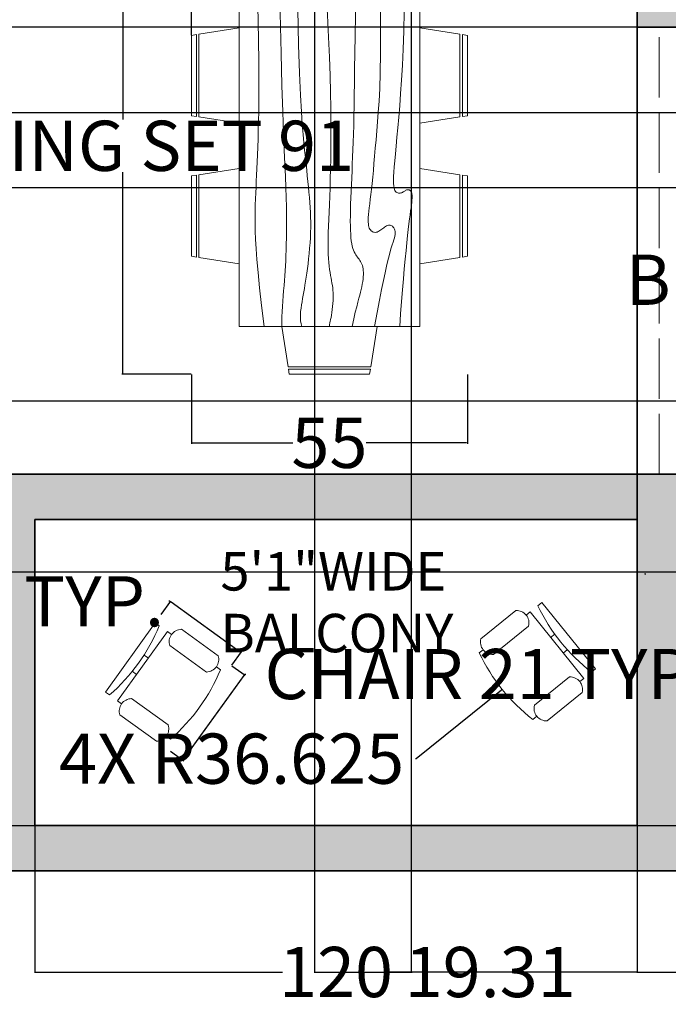
# Model space of a CAD drawing. Units: inches. Extents: x -75 to 484, y -248 to 214.
# Tile 4 of 7: x 162 to 291, y -248 to -52. Entities that reach past the tile are written whole.
import ezdxf

# ---------------------------------------------------------------- set-up
doc = ezdxf.new("R2010")
doc.units = ezdxf.units.IN
doc.header["$MEASUREMENT"] = 0
doc.linetypes.add('ACAD_ISO02W100', pattern=[15, 12, -3])
for name, color, linetype, lineweight in [('A-ANNO-DIMS', 2, 'Continuous', 18), ('A-AREA-IDEN', 7, 'Continuous', 18), ('A-FURN', 8, 'Continuous', 18), ('A-WALL', 7, 'Continuous', 35), ('A-WALL-OVHD', 7, 'ACAD_ISO02W100', 18)]:
    doc.layers.add(name, color=color, linetype=linetype, lineweight=lineweight)
doc.layers.add('A-WALL-PATT', color=252, linetype='Continuous', lineweight=9, true_color=0x939598)
doc.styles.get("Standard").update_dxf_attribs({"font": 'arial.ttf'})
doc.dimstyles.get("Standard").update_dxf_attribs({"dimtxt": 10, "dimasz": 0.18, "dimexe": 0.18, "dimexo": 0.0625, "dimgap": 0.09, "dimtad": 0, "dimtih": 1, "dimtoh": 1, "dimdec": 0, "dimzin": 0, "dimdsep": 46, "dimlunit": 3, "dimtxsty": 'Standard', "dimcen": 0.09, "dimadec": 0, "dimazin": 0, "dimtfac": 1, "dimtdec": 0, "dimtofl": 0, "dimtmove": 0, "dimatfit": 3, "dimfxl": 1, "dimtolj": 1, "dimtzin": 0, "dimarcsym": 0})

# ---------------------------------------------------------------- blocks, each defined once
blk = doc.blocks.new('Dining Set - 36 x 72 in.')
for p, q in [((-22, 27.5), (-22.1562, 26.50042)), ((-22, 27.5), (-6, 27.5)), ((-5.8437, 26.49966), (-6, 27.5)), ((6, 27.5), (5.8438, 26.50042)), ((6, 27.5), (22, 27.5)), ((22.1563, 26.49966), (22, 27.5)), ((-22.2343, 26.00059), (-23.4847, 17.99762)), ((-22.2304, 26), (-5.7608, 26)), ((-5.8416, 26.5), (-22.1534, 26.5)), ((-4.5152, 17.99762), (-5.7655, 25.99926)), ((5.7657, 26.00059), (4.5153, 17.99762)), ((5.7696, 26), (22.2392, 26)), ((22.1584, 26.5), (5.8466, 26.5)), ((23.4848, 17.99762), (22.2345, 25.99926)), ((36, 18), (-36, 18)), ((-36, 18), (-36, -18)), ((36, -18), (36, 18)), ((-45.5, 8), (-44.5004, 8.15617)), ((-45.5, 8), (-45.5, -8)), ((-44.5, -8.15843), (-44.5, 8.15338)), ((-44.0006, 8.23428), (-35.9976, 9.48474)), ((-44, 8.23041), (-44, -8.23915)), ((44.0006, 8.23428), (35.9976, 9.48474)), ((44, 8.23041), (44, -8.23915)), ((44.5, -8.15843), (44.5, 8.15338)), ((45.5, 8), (44.5005, 8.15617)), ((45.5, 8), (45.5, -8)), ((-44.4997, -8.15631), (-45.5, -8)), ((-35.9976, -9.48476), (-43.9993, -8.2345)), ((35.9976, -9.48476), (43.9993, -8.2345)), ((44.4997, -8.15631), (45.5, -8)), ((-36, -18), (36, -18)), ((-22.2343, -26.0006), (-23.4847, -17.99762)), ((-4.5152, -17.99762), (-5.7655, -25.99928)), ((5.7657, -26.0006), (4.5153, -17.99762)), ((23.4848, -17.99762), (22.2345, -25.99928)), ((-22.2304, -26), (-5.7608, -26)), ((-22, -27.5), (-22.1562, -26.50044)), ((-5.8416, -26.5), (-22.1534, -26.5)), ((-5.8437, -26.49967), (-6, -27.5)), ((5.7696, -26), (22.2392, -26)), ((6, -27.5), (5.8438, -26.50044)), ((22.1584, -26.5), (5.8466, -26.5)), ((22.1563, -26.49967), (22, -27.5)), ((-22, -27.5), (-6, -27.5)), ((6, -27.5), (22, -27.5))]:
    blk.add_line(p, q)
for points in [[(-36, 15), (-31.1772, 14.97754), (-26.8079, 14.91406), (-22.8538, 14.81543), (-19.276, 14.6875), (-16.0362, 14.53613), (-13.0957, 14.36718), (-10.4159, 14.18652), (-7.9583, 14), (-5.6904, 13.81315), (-3.6035, 13.63021), (-1.6954, 13.45508), (0.0365, 13.29166), (1.5945, 13.14388), (2.9811, 13.01562), (4.1988, 12.9108), (5.25, 12.83333), (6.1393, 12.78613), (6.8802, 12.76823), (7.4883, 12.77767), (7.9792, 12.8125), (8.3685, 12.87077), (8.6719, 12.95052), (8.9049, 13.0498), (9.0833, 13.16666), (9.2205, 13.29899), (9.3216, 13.44401), (9.3895, 13.59879), (9.4271, 13.76041), (9.4373, 13.92594), (9.4232, 14.09245), (9.3875, 14.257), (9.3333, 14.41666), (9.2638, 14.56917), (9.1836, 14.71484), (9.0975, 14.85465), (9.0104, 14.98958), (8.9272, 15.1206), (8.8529, 15.2487), (8.7922, 15.37483), (8.75, 15.5), (8.7305, 15.62467), (8.7344, 15.74739), (8.7617, 15.86621), (8.8125, 15.97916), (8.8867, 16.08431), (8.9844, 16.17968), (9.1055, 16.26334), (9.25, 16.33333), (9.4189, 16.38802), (9.6172, 16.42708), (9.8506, 16.45052), (10.125, 16.45833), (10.4463, 16.45052), (10.8203, 16.42708), (11.2529, 16.38802), (11.75, 16.33333), (12.3184, 16.26318), (12.9694, 16.17838), (13.7151, 16.07991), (14.5677, 15.96875), (15.5395, 15.84586), (16.6426, 15.71224), (17.8893, 15.56884), (19.2917, 15.41666), (20.859, 15.25667), (22.5879, 15.08984), (24.4721, 14.91715), (26.5052, 14.73958), (28.6809, 14.5581), (30.9929, 14.3737), (33.4347, 14.18733), (36, 14)], [(-36, 10), (-28.9766, 10.14274), (-23.1725, 10.20442), (-18.4241, 10.19775), (-14.5677, 10.13541), (-11.4399, 10.03011), (-8.877, 9.89453), (-6.7154, 9.74137), (-4.7917, 9.58333), (-2.9698, 9.43082), (-1.2246, 9.28515), (0.4415, 9.14534), (2.026, 9.01041), (3.5266, 8.87939), (4.9408, 8.7513), (6.266, 8.62516), (7.5, 8.5), (8.6411, 8.37549), (9.6914, 8.2539), (10.6538, 8.13818), (11.5312, 8.03125), (12.3267, 7.93603), (13.043, 7.85547), (13.6831, 7.79248), (14.25, 7.75), (14.7471, 7.7303), (15.1797, 7.73307), (15.5537, 7.75732), (15.875, 7.80208), (16.1494, 7.86637), (16.3828, 7.94922), (16.5811, 8.04964), (16.75, 8.16666), (16.8944, 8.29915), (17.0143, 8.44531), (17.1089, 8.60319), (17.1771, 8.77083), (17.218, 8.94629), (17.2305, 9.1276), (17.2137, 9.31282), (17.1667, 9.5), (17.0895, 9.6875), (16.987, 9.875), (16.8649, 10.0625), (16.7292, 10.25), (16.5856, 10.4375), (16.4401, 10.625), (16.2985, 10.8125), (16.1667, 11), (16.05, 11.18733), (15.9518, 11.3737), (15.8752, 11.5581), (15.8229, 11.73958), (15.798, 11.91715), (15.8034, 12.08984), (15.842, 12.25667), (15.9167, 12.41666), (16.0295, 12.56836), (16.1784, 12.70833), (16.3605, 12.83268), (16.5729, 12.9375), (16.8127, 13.01888), (17.0768, 13.07291), (17.3625, 13.0957), (17.6667, 13.08333), (17.9894, 13.03312), (18.3418, 12.94726), (18.7382, 12.82918), (19.1927, 12.68229), (19.7195, 12.51001), (20.3327, 12.31575), (21.0465, 12.10294), (21.875, 11.875), (22.8357, 11.63354), (23.959, 11.37304), (25.2786, 11.08618), (26.8282, 10.76562), (28.6414, 10.40405), (30.752, 9.99414), (33.1936, 9.52856), (36, 9)], [(-36, 5.5), (-30.7157, 5.3348), (-26.069, 5.20963), (-21.9946, 5.11767), (-18.4271, 5.05208), (-15.3009, 5.00602), (-12.5508, 4.97265), (-10.1112, 4.94515), (-7.9167, 4.91666), (-5.909, 4.88167), (-4.0586, 4.83984), (-2.3429, 4.79215), (-0.7396, 4.73958), (0.7739, 4.6831), (2.22, 4.6237), (3.6213, 4.56233), (5, 4.5), (6.373, 4.43782), (7.7344, 4.3776), (9.0723, 4.32129), (10.375, 4.27083), (11.6309, 4.22819), (12.8281, 4.19531), (13.9551, 4.17415), (15, 4.16666), (15.954, 4.17448), (16.819, 4.19791), (17.6001, 4.23698), (18.3021, 4.29166), (18.9299, 4.36198), (19.4883, 4.44791), (19.9823, 4.54948), (20.4167, 4.66666), (20.7969, 4.79899), (21.1302, 4.94401), (21.4245, 5.09879), (21.6875, 5.26041), (21.9271, 5.42594), (22.1511, 5.59245), (22.3672, 5.757), (22.5834, 5.91666), (22.8065, 6.06868), (23.0404, 6.21093), (23.2879, 6.34147), (23.5521, 6.45833), (23.8358, 6.55957), (24.142, 6.64323), (24.4735, 6.70735), (24.8334, 6.75), (25.2235, 6.76969), (25.642, 6.76692), (26.0858, 6.74267), (26.5521, 6.69791), (27.0379, 6.63362), (27.5404, 6.55078), (28.0565, 6.45036), (28.5834, 6.33333), (29.1242, 6.19987), (29.7071, 6.04687), (30.3661, 5.87044), (31.1354, 5.66666), (32.0493, 5.43164), (33.142, 5.16146), (34.4475, 4.85221), (36, 4.5)], [(-36, -1), (-30.7915, -0.6591), (-26.0195, -0.38216), (-21.6519, -0.16284), (-17.6563, 0.00521), (-14.0005, 0.12833), (-10.6523, 0.21289), (-7.5796, 0.26522), (-4.75, 0.29166), (-2.134, 0.29793), (0.2878, 0.28711), (2.5317, 0.26163), (4.6146, 0.22396), (6.5529, 0.17651), (8.3633, 0.12174), (10.0623, 0.06209), (11.6667, 0), (13.1899, -0.06201), (14.6341, -0.1211), (15.9982, -0.17432), (17.2813, -0.21875), (18.4823, -0.25147), (19.6003, -0.26953), (20.6343, -0.27002), (21.5834, -0.25), (22.4481, -0.20768), (23.2357, -0.14584), (23.9549, -0.06836), (24.6146, 0.02083), (25.2235, 0.11784), (25.7904, 0.21875), (26.3241, 0.31966), (26.8334, 0.41666), (27.3265, 0.50618), (27.8099, 0.58593), (28.2894, 0.65397), (28.7709, 0.70833), (29.2601, 0.74707), (29.763, 0.76823), (30.2855, 0.76985), (30.8334, 0.75), (31.4088, 0.70784), (31.9994, 0.64713), (32.589, 0.57275), (33.1615, 0.48958), (33.7008, 0.4025), (34.1908, 0.3164), (34.6153, 0.23616), (34.9584, 0.16666), (35.2099, 0.11165), (35.3848, 0.07031), (35.504, 0.04069), (35.5886, 0.02083), (35.6594, 0.00879), (35.7377, 0.0026), (35.8442, 0.00032), (36, 0)], [(-36, -6.5), (-27.1843, -6.31267), (-20.084, -6.1263), (-14.469, -5.9419), (-10.1094, -5.76042), (-6.7752, -5.58285), (-4.2363, -5.41016), (-2.2629, -5.24333), (-0.625, -5.08334), (0.8708, -4.93099), (2.2715, -4.78646), (3.5872, -4.64974), (4.8281, -4.52084), (6.0046, -4.39974), (7.127, -4.28646), (8.2053, -4.18099), (9.25, -4.08334), (10.2705, -3.99382), (11.2734, -3.91407), (12.2647, -3.84603), (13.25, -3.79167), (14.2354, -3.75293), (15.2266, -3.73177), (16.2295, -3.73015), (17.25, -3.75), (18.2912, -3.79248), (19.3451, -3.85547), (20.4009, -3.93604), (21.4479, -4.03125), (22.4754, -4.13819), (23.4727, -4.25391), (24.4289, -4.37549), (25.3334, -4.5), (26.1785, -4.62492), (26.9694, -4.74935), (27.7145, -4.87281), (28.4219, -4.99479), (29.1, -5.11483), (29.7572, -5.23242), (30.4016, -5.34709), (31.0417, -5.45834), (31.6837, -5.56437), (32.3262, -5.65821), (32.9658, -5.73153), (33.599, -5.77604), (34.2224, -5.78345), (34.8327, -5.74545), (35.4264, -5.65373), (36, -5.5)], [(-36, -10), (-26.4022, -9.81299), (-18.4675, -9.62891), (-11.9839, -9.45069), (-6.7396, -9.28125), (-2.5226, -9.12354), (0.8789, -8.98047), (3.6769, -8.85498), (6.0833, -8.75), (8.2767, -8.66765), (10.3021, -8.60677), (12.1712, -8.56543), (13.8958, -8.54167), (15.4876, -8.53353), (16.9583, -8.53907), (18.3197, -8.55632), (19.5834, -8.58334), (20.7616, -8.61841), (21.8685, -8.66081), (22.9188, -8.71004), (23.9271, -8.76563), (24.9081, -8.82707), (25.8763, -8.89388), (26.8465, -8.96558), (27.8334, -9.04167), (28.8474, -9.12118), (29.8828, -9.20117), (30.93, -9.27824), (31.9792, -9.34896), (33.0205, -9.40991), (34.0443, -9.45768), (35.0407, -9.48885), (36, -9.5)], [(-36, -14.5), (-30.0881, -14.33513), (-25.0332, -14.21224), (-20.7312, -14.12647), (-17.0781, -14.07292), (-13.97, -14.04671), (-11.3027, -14.04297), (-8.9724, -14.05681), (-6.875, -14.08334), (-4.9224, -14.11833), (-3.0905, -14.16016), (-1.3709, -14.20785), (0.2448, -14.26042), (1.7647, -14.3169), (3.1973, -14.3763), (4.5507, -14.43767), (5.8333, -14.5), (7.0554, -14.5621), (8.235, -14.62175), (9.3922, -14.67652), (10.5469, -14.72396), (11.7192, -14.76164), (12.929, -14.78711), (14.1965, -14.79794), (15.5417, -14.79167), (16.9933, -14.76424), (18.6152, -14.70508), (20.4804, -14.60197), (22.6615, -14.44271), (25.2312, -14.21509), (28.2624, -13.9069), (31.8277, -13.50594), (36, -13)]]:
    blk.add_lwpolyline(points)
blk = doc.blocks.new('Chair - Desk')
for p, q in [((-8.5, 0), (-8.5, -1)), ((-8.5, 0), (8.5, 0)), ((8.5, 0), (8.5, -1)), ((-2, -3), (-2, -1.9355)), ((2, -1.9576), (2, -3)), ((-8.5, -3), (-8.5, -4)), ((-8.5, -3), (8.5, -3)), ((8.5, -3), (8.5, -4)), ((-10.5, -5), (-10.5, -14)), ((-6.5, -14), (-6.5, -5)), ((6.5, -5), (6.5, -14)), ((10.5, -14), (10.5, -5)), ((-8.5, -15), (-8.5, -16)), ((8.5, -15), (8.5, -16))]:
    blk.add_line(p, q)
for centre, radius, start, end in [((0, 34.625), 36.625, 256.5803, 283.4197), ((-8.5, -6.5), 2.5, 36.8699, 143.1301), ((8.5, -6.5), 2.5, 36.8699, 143.1301), ((-8.5, -12.5), 2.5, 216.8699, 323.1301), ((8.5, -12.5), 2.5, 216.8699, 323.1301), ((0, 19.625), 36.625, 256.5803, 283.4197)]:
    blk.add_arc(centre, radius, start, end)
blk = doc.blocks.new('*D21')
at = {"layer": 'A-ANNO-DIMS', "color": 0, "lineweight": -2, "transparency": 16777216}
for p, q in [((204.49, -180.49), (207.14, -182.4)), ((207, -182.29), (207.1, -182.15)), ((207.1, -182.15), (207.28, -182.15)), ((194.83, -199.19), (206.89, -182.44)), ((192.22, -197.53), (194.87, -199.44))]:
    blk.add_line(p, q, dxfattribs=at)
at = {"layer": 'A-ANNO-DIMS', "color": 0, "transparency": 16777216}
for points in [[(206.87, -182.42), (206.92, -182.46), (207, -182.29)], [(194.8, -199.17), (194.85, -199.2), (194.72, -199.33)]]:
    blk.add_solid(points, dxfattribs=at)
at = {"layer": 'Defpoints', "color": 0, "transparency": 16777216}
for p in [(204.44, -180.45), (207, -182.29), (192.17, -197.49)]:
    blk.add_point(p, dxfattribs=at)
at = {"layer": 'A-ANNO-DIMS', "color": 0, "transparency": 16777216, "insert": (255.32, -182.15), "char_height": 10, "attachment_point": 5}
blk.add_mtext('\\A1;CHAIR 21 TYP.', dxfattribs=at)
blk = doc.blocks.new('*D22')
at = {"layer": 'A-ANNO-DIMS', "color": 0, "lineweight": -2, "transparency": 16777216}
for p, q in [((190.41, -170.27), (192.32, -167.62)), ((192.07, -167.66), (191.89, -167.66)), ((192.22, -167.77), (192.07, -167.66)), ((206.13, -177.79), (192.36, -167.87)), ((204.48, -180.4), (206.39, -177.75))]:
    blk.add_line(p, q, dxfattribs=at)
at = {"layer": 'A-ANNO-DIMS', "color": 0, "transparency": 16777216}
for points in [[(192.38, -167.85), (192.34, -167.89), (192.22, -167.77)], [(206.15, -177.77), (206.12, -177.81), (206.28, -177.9)]]:
    blk.add_solid(points, dxfattribs=at)
at = {"layer": 'Defpoints', "color": 0, "transparency": 16777216}
for p in [(192.22, -167.77), (190.37, -170.32), (204.44, -180.45)]:
    blk.add_point(p, dxfattribs=at)
at = {"layer": 'A-ANNO-DIMS', "color": 0, "transparency": 16777216, "insert": (167.93, -167.66), "char_height": 10, "attachment_point": 5}
blk.add_mtext('\\A1;17 TYP.', dxfattribs=at)
blk = doc.blocks.new('*D27')
at = {"layer": 'A-ANNO-DIMS', "color": 0, "lineweight": -2, "transparency": 16777216}
for p, q in [((196.34, -31.46), (182.57, -31.46)), ((182.75, -31.64), (182.75, -71.7)), ((182.75, -122.28), (182.75, -82.22)), ((196.34, -122.46), (182.57, -122.46))]:
    blk.add_line(p, q, dxfattribs=at)
at = {"layer": 'A-ANNO-DIMS', "color": 0, "transparency": 16777216}
for points in [[(182.72, -31.64), (182.78, -31.64), (182.75, -31.46)], [(182.72, -122.28), (182.78, -122.28), (182.75, -122.46)]]:
    blk.add_solid(points, dxfattribs=at)
at = {"layer": 'Defpoints', "color": 0, "transparency": 16777216}
for p in [(196.4, -31.46), (182.75, -122.46), (196.4, -122.46)]:
    blk.add_point(p, dxfattribs=at)
at = {"layer": 'A-ANNO-DIMS', "color": 0, "transparency": 16777216, "insert": (182.75, -76.96), "char_height": 10, "attachment_point": 5}
blk.add_mtext('\\A1;DINING SET 91', dxfattribs=at)
blk = doc.blocks.new('*D28')
at = {"layer": 'A-ANNO-DIMS', "color": 0, "lineweight": -2, "transparency": 16777216}
for p, q in [((196.4, -122.53), (196.4, -136.29)), ((251.4, -122.53), (251.4, -136.29)), ((196.58, -136.11), (216.61, -136.11)), ((251.22, -136.11), (231.19, -136.11))]:
    blk.add_line(p, q, dxfattribs=at)
at = {"layer": 'A-ANNO-DIMS', "color": 0, "transparency": 16777216}
for points in [[(196.58, -136.08), (196.58, -136.14), (196.4, -136.11)], [(251.22, -136.08), (251.22, -136.14), (251.4, -136.11)]]:
    blk.add_solid(points, dxfattribs=at)
at = {"layer": 'Defpoints', "color": 0, "transparency": 16777216}
for p in [(196.4, -122.46), (251.4, -122.46), (251.4, -136.11)]:
    blk.add_point(p, dxfattribs=at)
at = {"layer": 'A-ANNO-DIMS', "color": 0, "transparency": 16777216, "insert": (223.9, -136.11), "char_height": 10, "attachment_point": 5}
blk.add_mtext('\\A1;55', dxfattribs=at)
blk = doc.blocks.new('*D37')
at = {"layer": 'A-ANNO-DIMS', "color": 0, "lineweight": -2, "transparency": 16777216}
for p, q in [((390.31, -103.63), (390.13, -103.63)), ((390.31, -105.1), (390.31, -103.45)), ((400.34, -103.63), (390.49, -103.63)), ((400.52, -105.1), (400.52, -103.45))]:
    blk.add_line(p, q, dxfattribs=at)
at = {"layer": 'A-ANNO-DIMS', "color": 0, "transparency": 16777216}
for points in [[(390.49, -103.6), (390.49, -103.66), (390.31, -103.63)], [(400.34, -103.6), (400.34, -103.66), (400.52, -103.63)]]:
    blk.add_solid(points, dxfattribs=at)
at = {"layer": 'Defpoints', "color": 0, "transparency": 16777216}
for p in [(390.31, -103.63), (390.31, -105.16), (400.52, -105.16)]:
    blk.add_point(p, dxfattribs=at)
at = {"layer": 'A-ANNO-DIMS', "color": 0, "transparency": 16777216, "insert": (334.48, -103.63), "char_height": 10, "attachment_point": 5}
blk.add_mtext('\\A1;BURNER 10 TYP.', dxfattribs=at)
blk = doc.blocks.new('*D43')
at = {"layer": 'A-ANNO-DIMS', "color": 0, "lineweight": -2, "transparency": 16777216}
for p, q in [((220.9, 147.59), (220.9, -241.67)), ((240.21, 138.59), (240.21, -241.67)), ((221.08, -241.49), (240.03, -241.49)), ((240.21, -241.49), (240.39, -241.49))]:
    blk.add_line(p, q, dxfattribs=at)
at = {"layer": 'A-ANNO-DIMS', "color": 0, "transparency": 16777216}
for points in [[(221.08, -241.46), (221.08, -241.52), (220.9, -241.49)], [(240.03, -241.46), (240.03, -241.52), (240.21, -241.49)]]:
    blk.add_solid(points, dxfattribs=at)
at = {"layer": 'Defpoints', "color": 0, "transparency": 16777216}
for p in [(220.9, 147.66), (240.21, 138.66), (240.21, -241.49)]:
    blk.add_point(p, dxfattribs=at)
at = {"layer": 'A-ANNO-DIMS', "color": 0, "transparency": 16777216, "insert": (255.92, -241.49), "char_height": 10, "attachment_point": 5}
blk.add_mtext('\\A1;19.31', dxfattribs=at)
blk = doc.blocks.new('*D56')
at = {"layer": 'A-ANNO-DIMS', "color": 0, "lineweight": -2, "transparency": 16777216}
for p, q in [((165.21, -212.41), (165.21, -241.67)), ((285.21, -212.41), (285.21, -241.67)), ((165.39, -241.49), (214.56, -241.49)), ((285.03, -241.49), (235.86, -241.49))]:
    blk.add_line(p, q, dxfattribs=at)
at = {"layer": 'A-ANNO-DIMS', "color": 0, "transparency": 16777216}
for points in [[(165.39, -241.46), (165.39, -241.52), (165.21, -241.49)], [(285.03, -241.46), (285.03, -241.52), (285.21, -241.49)]]:
    blk.add_solid(points, dxfattribs=at)
at = {"layer": 'Defpoints', "color": 0, "transparency": 16777216}
for p in [(165.21, -212.34), (285.21, -212.34), (285.21, -241.49)]:
    blk.add_point(p, dxfattribs=at)
at = {"layer": 'A-ANNO-DIMS', "color": 0, "transparency": 16777216, "insert": (225.21, -241.49), "char_height": 10, "attachment_point": 5}
blk.add_mtext('\\A1;120', dxfattribs=at)
blk = doc.blocks.new('*D57')
at = {"layer": 'A-ANNO-DIMS', "color": 0, "lineweight": -2, "transparency": 16777216}
for p, q in [((285.21, -212.28), (285.21, 167.99)), ((285.39, 167.81), (285.82, 167.81)), ((293.03, 167.81), (292.59, 167.81)), ((293.21, -212.28), (293.21, 167.99))]:
    blk.add_line(p, q, dxfattribs=at)
at = {"layer": 'A-ANNO-DIMS', "color": 0, "transparency": 16777216}
for points in [[(285.39, 167.84), (285.39, 167.78), (285.21, 167.81)], [(293.03, 167.84), (293.03, 167.78), (293.21, 167.81)]]:
    blk.add_solid(points, dxfattribs=at)
at = {"layer": 'Defpoints', "color": 0, "transparency": 16777216}
for p in [(285.21, 167.81), (285.21, -212.34), (293.21, -212.34)]:
    blk.add_point(p, dxfattribs=at)
at = {"layer": 'A-ANNO-DIMS', "color": 0, "transparency": 16777216, "insert": (289.21, 167.81), "char_height": 10, "attachment_point": 5}
blk.add_mtext('\\A1;8', dxfattribs=at)
blk = doc.blocks.new('*D67')
at = {"layer": 'A-ANNO-DIMS', "color": 0, "lineweight": -2, "transparency": 16777216}
for p, q in [((325.99, -53.34), (-5.12, -53.34)), ((-4.94, -53.52), (-4.94, -56.68)), ((-4.94, -70.23), (-4.94, -67.07)), ((325.99, -70.41), (-5.12, -70.41))]:
    blk.add_line(p, q, dxfattribs=at)
at = {"layer": 'A-ANNO-DIMS', "color": 0, "transparency": 16777216}
for points in [[(-4.97, -53.52), (-4.91, -53.52), (-4.94, -53.34)], [(-4.97, -70.23), (-4.91, -70.23), (-4.94, -70.41)]]:
    blk.add_solid(points, dxfattribs=at)
at = {"layer": 'Defpoints', "color": 0, "transparency": 16777216}
for p in [(326.06, -53.34), (-4.94, -70.41), (326.06, -70.41)]:
    blk.add_point(p, dxfattribs=at)
at = {"layer": 'A-ANNO-DIMS', "color": 0, "transparency": 16777216, "insert": (-4.94, -61.88), "char_height": 10, "attachment_point": 5}
blk.add_mtext('\\A1;17.068', dxfattribs=at)
blk = doc.blocks.new('*D68')
at = {"layer": 'A-ANNO-DIMS', "color": 0, "lineweight": -2, "transparency": 16777216}
for p, q in [((340.8, -127.84), (-5.12, -127.84)), ((-4.94, -128.02), (-4.94, -129.9)), ((-4.94, -142.16), (-4.94, -140.29)), ((340.8, -142.34), (-5.12, -142.34))]:
    blk.add_line(p, q, dxfattribs=at)
at = {"layer": 'A-ANNO-DIMS', "color": 0, "transparency": 16777216}
for points in [[(-4.97, -128.02), (-4.91, -128.02), (-4.94, -127.84)], [(-4.97, -142.16), (-4.91, -142.16), (-4.94, -142.34)]]:
    blk.add_solid(points, dxfattribs=at)
at = {"layer": 'Defpoints', "color": 0, "transparency": 16777216}
for p in [(340.87, -127.84), (-4.94, -142.34), (340.87, -142.34)]:
    blk.add_point(p, dxfattribs=at)
at = {"layer": 'A-ANNO-DIMS', "color": 0, "transparency": 16777216, "insert": (-4.94, -135.09), "char_height": 10, "attachment_point": 5}
blk.add_mtext('\\A1;14.5', dxfattribs=at)
blk = doc.blocks.new('*D69')
at = {"layer": 'A-ANNO-DIMS', "color": 0, "lineweight": -2, "transparency": 16777216}
for p, q in [((285.15, -53.34), (-5.12, -53.34)), ((-4.94, -53.52), (-4.94, -92.65)), ((-4.94, -142.16), (-4.94, -103.04)), ((285.15, -142.34), (-5.12, -142.34))]:
    blk.add_line(p, q, dxfattribs=at)
at = {"layer": 'A-ANNO-DIMS', "color": 0, "transparency": 16777216}
for points in [[(-4.97, -53.52), (-4.91, -53.52), (-4.94, -53.34)], [(-4.97, -142.16), (-4.91, -142.16), (-4.94, -142.34)]]:
    blk.add_solid(points, dxfattribs=at)
at = {"layer": 'Defpoints', "color": 0, "transparency": 16777216}
for p in [(285.21, -53.34), (-4.94, -142.34), (285.21, -142.34)]:
    blk.add_point(p, dxfattribs=at)
at = {"layer": 'A-ANNO-DIMS', "color": 0, "transparency": 16777216, "insert": (-4.94, -97.84), "char_height": 10, "attachment_point": 5}
blk.add_mtext('\\A1;89', dxfattribs=at)
blk = doc.blocks.new('*D70')
at = {"layer": 'A-ANNO-DIMS', "color": 0, "lineweight": -2, "transparency": 16777216}
for p, q in [((285.21, -53.41), (285.21, -241.67)), ((405.21, -53.41), (405.21, -241.67)), ((285.39, -241.49), (334.56, -241.49)), ((405.03, -241.49), (355.86, -241.49))]:
    blk.add_line(p, q, dxfattribs=at)
at = {"layer": 'A-ANNO-DIMS', "color": 0, "transparency": 16777216}
for points in [[(285.39, -241.46), (285.39, -241.52), (285.21, -241.49)], [(405.03, -241.46), (405.03, -241.52), (405.21, -241.49)]]:
    blk.add_solid(points, dxfattribs=at)
at = {"layer": 'Defpoints', "color": 0, "transparency": 16777216}
for p in [(285.21, -53.34), (405.21, -53.34), (405.21, -241.49)]:
    blk.add_point(p, dxfattribs=at)
at = {"layer": 'A-ANNO-DIMS', "color": 0, "transparency": 16777216, "insert": (345.21, -241.49), "char_height": 10, "attachment_point": 5}
blk.add_mtext('\\A1;120', dxfattribs=at)
blk = doc.blocks.new('*D72')
at = {"layer": 'A-ANNO-DIMS', "color": 0, "lineweight": -2, "transparency": 16777216}
for p, q in [((382.5, -70.41), (-5.12, -70.41)), ((-4.94, -70.59), (-4.94, -72.68)), ((-4.94, -85.15), (-4.94, -83.07)), ((382.5, -85.33), (-5.12, -85.33))]:
    blk.add_line(p, q, dxfattribs=at)
at = {"layer": 'A-ANNO-DIMS', "color": 0, "transparency": 16777216}
for points in [[(-4.97, -70.59), (-4.91, -70.59), (-4.94, -70.41)], [(-4.97, -85.15), (-4.91, -85.15), (-4.94, -85.33)]]:
    blk.add_solid(points, dxfattribs=at)
at = {"layer": 'Defpoints', "color": 0, "transparency": 16777216}
for p in [(382.57, -70.41), (-4.94, -85.33), (382.57, -85.33)]:
    blk.add_point(p, dxfattribs=at)
at = {"layer": 'A-ANNO-DIMS', "color": 0, "transparency": 16777216, "insert": (-4.94, -77.87), "char_height": 10, "attachment_point": 5}
blk.add_mtext('\\A1;14.92', dxfattribs=at)
blk = doc.blocks.new('*D74')
at = {"layer": 'A-ANNO-DIMS', "color": 0, "lineweight": -2, "transparency": 16777216}
for p, q in [((24.27, -161.82), (434.54, -161.82)), ((434.36, -162), (434.36, -181.88)), ((434.36, -212.16), (434.36, -192.28)), ((24.27, -212.34), (434.54, -212.34))]:
    blk.add_line(p, q, dxfattribs=at)
at = {"layer": 'A-ANNO-DIMS', "color": 0, "transparency": 16777216}
for points in [[(434.33, -162), (434.39, -162), (434.36, -161.82)], [(434.33, -212.16), (434.39, -212.16), (434.36, -212.34)]]:
    blk.add_solid(points, dxfattribs=at)
at = {"layer": 'Defpoints', "color": 0, "transparency": 16777216}
for p in [(24.21, -161.82), (434.36, -161.82), (24.21, -212.34)]:
    blk.add_point(p, dxfattribs=at)
at = {"layer": 'A-ANNO-DIMS', "color": 0, "transparency": 16777216, "insert": (434.36, -187.08), "char_height": 10, "attachment_point": 5}
blk.add_mtext('\\A1;50.53', dxfattribs=at)
blk = doc.blocks.new('*D77')
at = {"layer": 'A-ANNO-DIMS', "color": 0, "lineweight": -2, "transparency": 16777216}
for p, q in [((159.21, -53.28), (159.21, 167.99)), ((159.39, 167.81), (160.83, 167.81)), ((196.22, 167.81), (194.77, 167.81)), ((196.4, -54.9), (196.4, 167.99))]:
    blk.add_line(p, q, dxfattribs=at)
at = {"layer": 'A-ANNO-DIMS', "color": 0, "transparency": 16777216}
for points in [[(159.39, 167.84), (159.39, 167.78), (159.21, 167.81)], [(196.22, 167.84), (196.22, 167.78), (196.4, 167.81)]]:
    blk.add_solid(points, dxfattribs=at)
at = {"layer": 'Defpoints', "color": 0, "transparency": 16777216}
for p in [(196.4, 167.81), (159.21, -53.34), (196.4, -54.96)]:
    blk.add_point(p, dxfattribs=at)
at = {"layer": 'A-ANNO-DIMS', "color": 0, "transparency": 16777216, "insert": (177.8, 167.81), "char_height": 10, "attachment_point": 5}
blk.add_mtext('\\A1;37.19', dxfattribs=at)
blk = doc.blocks.new('*D89')
at = {"layer": 'A-ANNO-DIMS', "color": 0, "lineweight": -2, "transparency": 16777216}
for p, q in [((286.72, -162.2), (286.9, -162.2)), ((286.81, -162.29), (286.81, -162.11)), ((241.21, -199), (258.17, -185.31)), ((241.03, -199), (241.21, -199))]:
    blk.add_line(p, q, dxfattribs=at)
at = {"layer": 'A-ANNO-DIMS', "color": 0, "transparency": 16777216}
blk.add_solid([(258.15, -185.29), (258.19, -185.33), (258.31, -185.2)], dxfattribs=at)
at = {"layer": 'Defpoints', "color": 0, "transparency": 16777216}
for p in [(286.81, -162.2), (258.31, -185.2)]:
    blk.add_point(p, dxfattribs=at)
at = {"layer": 'A-ANNO-DIMS', "color": 0, "transparency": 16777216, "insert": (204.41, -199), "char_height": 10, "attachment_point": 5}
blk.add_mtext('\\A1;4X R36.625', dxfattribs=at)

msp = doc.modelspace()

# ---------------------------------------------------------------- hatches: boundary and pattern name
at = {"layer": 'A-WALL-PATT'}
h = msp.add_hatch(color=256, dxfattribs=at)
h.dxf.hatch_style = 1
h.paths.add_polyline_path([(184.9004, 147.6567), (15.2094, 147.6567), (15.2094, 92.5031), (24.2094, 92.5031), (24.2094, 138.6567), (186.0436, 138.6567, -0.06325422)])
h.paths.add_polyline_path([(414.2094, 147.6567), (249.2094, 147.6567), (220.9004, 147.6567), (220.9004, 138.6567), (240.2094, 138.6567), (240.2094, 18.6567), (240.2094, 9.6567), (249.2094, 9.6567), (249.2094, 45.6567), (249.2094, 138.6567), (405.2094, 138.6567), (405.2094, 98.3029), (414.2094, 98.3029)])
h.paths.add_polyline_path([(159.2094, 18.6567), (24.2094, 18.6567), (24.2094, 44.5861), (15.2094, 44.5861), (15.2094, 9.6567), (15.2094, -3.1791), (24.2094, -3.1791), (24.2094, 9.6567), (132.2094, 9.6567), (132.2094, -50.3433), (83.7394, -50.3433), (83.7394, -53.3433), (132.2094, -53.3433), (159.2094, -53.3433), (159.2094, -50.3433), (135.2094, -50.3433), (135.2094, 9.6567), (159.2094, 9.6567)])
h.paths.add_polyline_path([(53.8898, -50.3433), (24.2094, -50.3433), (24.2094, -27.303), (15.2094, -27.303), (15.2094, -50.3433), (15.2094, -53.3433), (15.2094, -74.0487), (24.2094, -74.0487), (24.2094, -53.3433), (53.7394, -53.3433, -0.02504709)])
h.paths.add_polyline_path([(24.2094, -121.9657), (15.2094, -121.9657), (15.2094, -212.3433), (15.2094, -221.3433), (24.2094, -221.3433), (84.3017, -221.3433), (84.3017, -212.3433), (24.2094, -212.3433)])
h.paths.add_polyline_path([(414.2094, -155.3433), (414.2094, -53.3433), (414.2094, -50.3433), (414.2094, -36.8417), (405.2094, -36.8417), (405.2094, -50.3433), (309.2094, -50.3433), (309.2094, 16.0463), (324.2573, 16.0463), (324.2573, 18.6567), (284.0663, 18.6567, -0.06325422), (285.2094, 9.6567), (306.2094, 9.6567), (306.2094, -50.3433), (285.2094, -50.3433), (285.2094, -53.3433), (309.2094, -53.3433), (405.2094, -53.3433), (405.2094, -212.3433), (293.2094, -212.3433), (293.2094, -158.3433), (293.2094, -145.3433), (300.0339, -145.3433), (300.0339, -142.3433), (285.2094, -142.3433), (159.2094, -142.3433), (159.2094, -89.3433, -0.02086055), (156.2094, -89.218), (156.2094, -212.3433), (131.9001, -212.3433), (131.9001, -221.3433), (156.2094, -221.3433), (165.2094, -221.3433), (285.2094, -221.3433), (288.6713, -221.3433), (293.2094, -221.3433), (405.2094, -221.3433), (414.2094, -221.3433)])
h.paths.add_polyline_path([(165.2094, -212.3433), (165.2094, -151.3433), (285.2094, -151.3433), (285.2094, -212.3433)], flags=16)
h.paths.add_polyline_path([(189.462, -195.5437), (182.159, -190.2838, -0.23606798), (182.5164, -188.0765), (181.7049, -187.4921), (185.5037, -182.2177), (184.648, -181.6013, -0.04492589), (180.0821, -186.3232), (179.2706, -185.7388), (189.206, -171.9443), (190.0174, -172.5287, -0.04492589), (186.9857, -178.3556), (187.8415, -178.9719), (191.6403, -173.6976), (192.4517, -174.282, -0.23606798), (194.432, -173.2435), (201.735, -178.5034, -0.23606798), (201.3776, -180.7107), (202.189, -181.2952, -0.11764706), (192.2537, -195.0897), (191.4423, -194.5053, -0.23606798)], flags=0)
h.paths.add_polyline_path([(253.751, -177.9543), (254.5293, -177.3263, -0.23606798), (254.0517, -175.1419), (261.056, -169.4904, -0.23606798), (263.0902, -170.419), (263.8684, -169.7911), (267.95, -174.8498), (268.7708, -174.1875, -0.04492589), (265.425, -168.5352), (266.2032, -167.9073), (276.8782, -181.1378), (276.0999, -181.7657, -0.04492589), (271.2826, -177.3006), (270.4618, -177.9629), (274.5434, -183.0216), (273.7651, -183.6495, -0.23606798), (274.2427, -185.834), (267.2383, -191.4854, -0.23606798), (265.2042, -190.5568), (264.4259, -191.1848, -0.11764706)], flags=0)
h.paths.add_polyline_path([(405.2094, -142.3433), (336.0339, -142.3433, -0.02086055), (335.9087, -145.3433), (405.2094, -145.3433)], flags=17)
h.paths.add_polyline_path([(414.2094, 50.4831), (405.2094, 50.4831), (405.2094, 18.6567), (354.2573, 18.6567, -0.02178446), (354.1435, 16.0463), (405.2094, 16.0463), (405.2094, -14.6494), (414.2094, -14.6494), (414.2094, 9.6567)])
h.paths.add_polyline_path([(200.2091, -179.9247), (255.2702, -179.9247), (255.2702, -168.0448), (200.2091, -168.0448)], flags=8)
h.paths.add_polyline_path([(200.2352, -167.6036), (249.7883, -167.6036), (249.7883, -155.8804), (200.2352, -155.8804)], flags=8)

# ---------------------------------------------------------------- linework, layer by layer
at = {"layer": 'A-WALL'}
for p, q in [((285.2094, -53.3433), (285.2094, -50.3433)), ((309.2094, -53.3433), (285.2094, -53.3433)), ((159.2094, -142.3433), (285.2094, -142.3433)), ((301.0339, -142.3433), (285.2094, -142.3433)), ((165.2094, -212.3433), (165.2094, -151.3433)), ((165.2094, -212.3433), (165.2094, -151.3433)), ((165.2094, -151.3433), (285.2094, -151.3433)), ((285.2094, -212.3433), (285.2094, -151.3433)), ((165.2094, -212.3433), (285.2094, -212.3433)), ((165.2094, -221.3433), (156.2094, -221.3433)), ((165.2094, -221.3433), (285.2094, -221.3433)), ((288.6713, -221.3433), (285.2094, -221.3433)), ((293.2094, -221.3433), (288.6713, -221.3433))]:
    msp.add_line(p, q, dxfattribs=at)
at = {"layer": 'A-WALL-OVHD'}
for p, q in [((285.2094, -53.3433), (285.2094, -142.3433)), ((289.5879, -142.3433), (289.5879, -53.3433))]:
    msp.add_line(p, q, dxfattribs=at)

# ---------------------------------------------------------------- block references
at = {"layer": 'A-FURN'}
for name, p, rotation in [('Dining Set - 36 x 72 in.', (223.8986, -76.9627), 270), ('Chair - Desk', (271.5407, -174.5225), 308.898047643191), ('Chair - Desk', (184.2383, -178.8415), 54.23714551867042)]:
    msp.add_blockref(name, p, dxfattribs=dict(at, rotation=rotation))

# ---------------------------------------------------------------- texts
at = {"layer": 'A-AREA-IDEN'}
for s, p in [('5\'1"WIDE', (202.189, -165.5192)), ('BALCONY', (202.189, -177.8142))]:
    msp.add_text(s, height=7.65368, dxfattribs=at).set_placement(p)

# ---------------------------------------------------------------- dimensions: what is measured, and where the dimension line sits
at = {"layer": 'A-ANNO-DIMS'}
for base, p1, p2, override, picture, middle in [((196.3986, 167.8067), (159.2094, -53.3433), (196.3986, -54.9627), {"dimdec": 2, "dimlfac": 1, "dimrnd": 0, "dimzin": 0, "dimdsep": 46, "dimlunit": 2}, '*D77', (177.804, 167.8067)), ((285.2094, 167.8067), (293.2094, -212.3433), (285.2094, -212.3433), {"dimdec": 0, "dimlfac": 1, "dimrnd": 0, "dimzin": 0, "dimdsep": 46, "dimlunit": 2}, '*D57', (289.2094, 167.8067)), ((240.2094, -241.4933), (220.9004, 147.6567), (240.2094, 138.6567), {"dimdec": 2, "dimlfac": 1, "dimrnd": 0, "dimzin": 0, "dimdsep": 46, "dimlunit": 2}, '*D43', (255.916, -241.4933)), ((405.2094, -241.4933), (285.2094, -53.3433), (405.2094, -53.3433), {"dimdec": 0, "dimlfac": 1, "dimrnd": 0, "dimzin": 0, "dimdsep": 46, "dimlunit": 2}, '*D70', (345.2094, -241.4933)), ((251.3986, -136.1127), (196.3986, -122.4627), (251.3986, -122.4627), {"dimdec": 0, "dimlfac": 1, "dimrnd": 0, "dimzin": 0, "dimdsep": 46, "dimlunit": 2}, '*D28', (223.8986, -136.1127)), ((285.2094, -241.4933), (165.2094, -212.3433), (285.2094, -212.3433), {"dimdec": 0, "dimlfac": 1, "dimrnd": 0, "dimzin": 0, "dimdsep": 46, "dimlunit": 2}, '*D56', (225.2094, -241.4933))]:
    dim = msp.add_linear_dim(base=base, p1=p1, p2=p2, dimstyle='Standard', override=override, dxfattribs=at)
    dim.commit()
    dim.dimension.update_dxf_attribs({"geometry": picture, "text_midpoint": middle})
for base, p1, p2, angle, text, picture, middle in [((182.7486, -122.4627), (196.3986, -31.4627), (196.3986, -122.4627), 270, 'DINING SET <>', '*D27', (182.7486, -76.9627)), ((390.3065, -103.6302), (400.5232, -105.1627), (390.3065, -105.1627), 180, 'BURNER <> TYP.', '*D37', (334.484, -103.6302)), ((192.2158, -167.7653), (204.4398, -180.4515), (190.3748, -170.3214), 144.237146, '<> TYP.', '*D22', (167.932, -167.6601)), ((206.9959, -182.2925), (192.1668, -197.4918), (204.4398, -180.4515), 54.237146, 'CHAIR <> TYP.', '*D21', (255.3247, -182.1464))]:
    dim = msp.add_linear_dim(base=base, p1=p1, p2=p2, angle=angle, text=text, dimstyle='Standard', override={"dimdec": 0, "dimlfac": 1, "dimrnd": 0, "dimzin": 0, "dimdsep": 46, "dimlunit": 2}, dxfattribs=at)
    dim.commit()
    dim.dimension.update_dxf_attribs({"geometry": picture, "text_midpoint": middle})
for base, p1, p2, override, picture, middle in [((-4.9406, -70.4114), (326.0553, -53.3433), (326.0553, -70.4114), {"dimdec": 3, "dimlfac": 1, "dimrnd": 0, "dimzin": 0, "dimdsep": 46, "dimlunit": 2}, '*D67', (-4.9406, -61.8773)), ((-4.9406, -142.3433), (285.2094, -53.3433), (285.2094, -142.3433), {"dimdec": 0, "dimlfac": 1, "dimrnd": 0, "dimzin": 0, "dimdsep": 46, "dimlunit": 2}, '*D69', (-4.9406, -97.8433)), ((-4.9406, -85.3314), (382.5668, -70.4114), (382.5668, -85.3314), {"dimdec": 2, "dimlfac": 1, "dimrnd": 0, "dimzin": 0, "dimdsep": 46, "dimlunit": 2}, '*D72', (-4.9406, -77.8714)), ((-4.9406, -142.3433), (340.8661, -127.8437), (340.8661, -142.3433), {"dimdec": 1, "dimlfac": 1, "dimrnd": 0, "dimzin": 0, "dimdsep": 46, "dimlunit": 2}, '*D68', (-4.9406, -135.0935)), ((434.3594, -161.8152), (24.2094, -212.3433), (24.2094, -161.8152), {"dimdec": 2, "dimlfac": 1, "dimrnd": 0, "dimzin": 0, "dimdsep": 46, "dimlunit": 2}, '*D74', (434.3594, -187.0792))]:
    dim = msp.add_linear_dim(base=base, p1=p1, p2=p2, angle=90, dimstyle='Standard', override=override, dxfattribs=at)
    dim.commit()
    dim.dimension.update_dxf_attribs({"geometry": picture, "text_midpoint": middle})
dim = msp.add_radius_dim(center=(286.8141, -162.1993), mpoint=(258.3099, -185.1971), text='4X <>', dimstyle='Standard', override={"dimdec": 3, "dimlfac": 1, "dimrnd": 0, "dimzin": 0, "dimdsep": 46, "dimlunit": 2}, dxfattribs=at)
dim.commit()
dim.dimension.update_dxf_attribs({"geometry": '*D89', "text_midpoint": (204.4128, -198.9958), "dimtype": 164})

doc.saveas('drawing.dxf')
